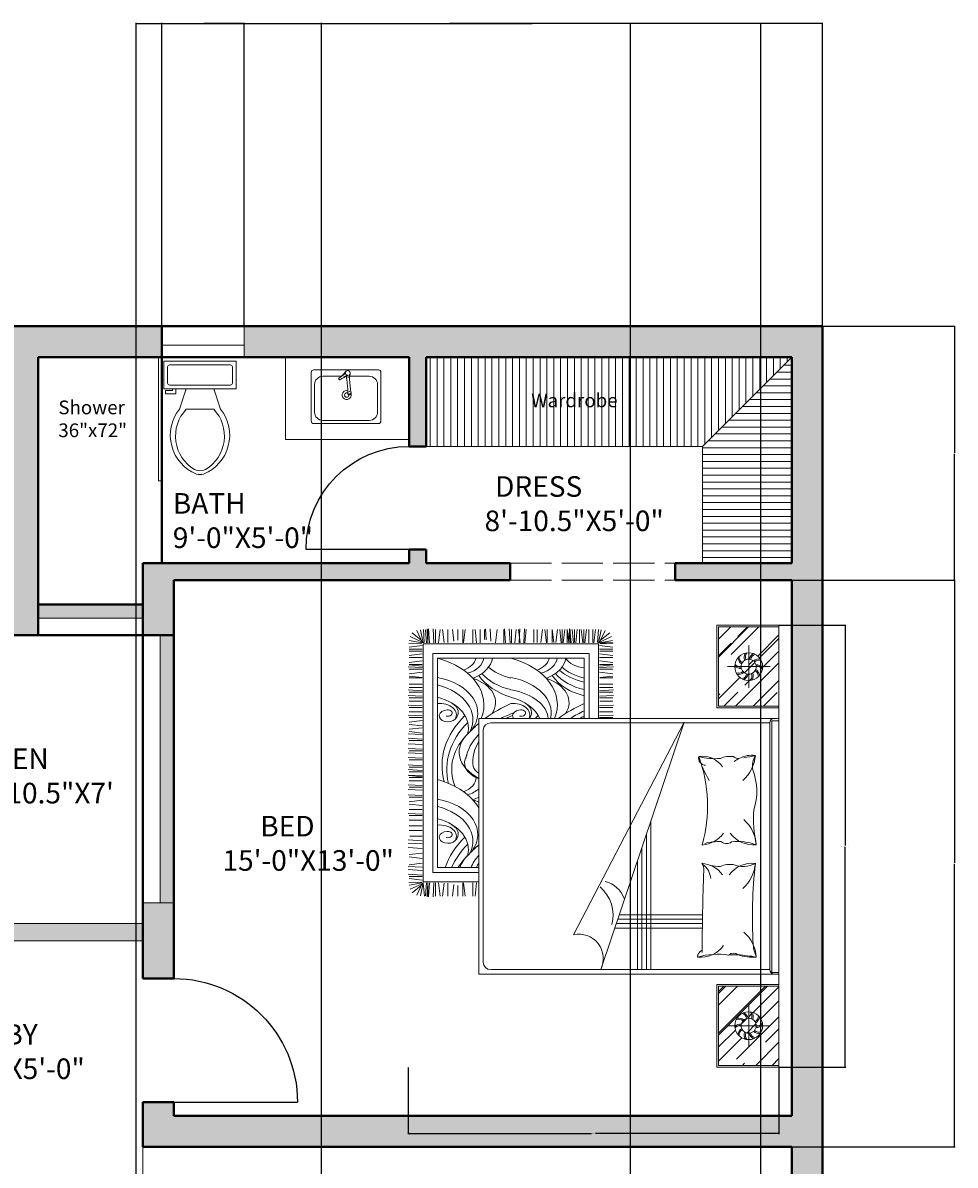
# Model space of a CAD drawing. Units: inches. Extents: x 2985 to 3527, y 3685 to 4528.
# Tile 5 of 5: x 3255 to 3527, y 4195 to 4528. Entities that reach past the tile are written whole.
import ezdxf

# ---------------------------------------------------------------- set-up
doc = ezdxf.new("R2010")
doc.units = ezdxf.units.IN
doc.linetypes.add('ACAD_ISO02W100', pattern=[15, 12, -3])
for name, color, linetype, lineweight in [('A-ANNO-DIMS', 2, 'Continuous', 18), ('A-ANNO-TEXT', 7, 'Continuous', 18), ('A-AREA-IDEN', 7, 'Continuous', 25), ('A-FLOR-CASE', 9, 'Continuous', 20), ('A-FLOR-CASE-PATT', 9, 'Continuous', 13), ('A-FLOR-FIXT', 9, 'Continuous', 18), ('A-FURN', 8, 'Continuous', 18), ('A-GLAZ', 4, 'Continuous', 18), ('A-WALL', 7, 'Continuous', 40), ('A-WALL-OVHD', 7, 'ACAD_ISO02W100', 18), ('A-WALL-PATT', 8, 'Continuous', 13), ('door', 4, 'Continuous', 25)]:
    doc.layers.add(name, color=color, linetype=linetype, lineweight=lineweight)
doc.layers.add('A-GLAZ-PATT', color=241, linetype='Continuous', lineweight=13, true_color=0xf7abae)
doc.styles.get("Standard").update_dxf_attribs({"font": 'arial.ttf'})
doc.dimstyles.get("Standard").update_dxf_attribs({"dimtxt": 0.18, "dimasz": 0.18, "dimexe": 0.18, "dimexo": 0.0625, "dimgap": 0.09, "dimtad": 0, "dimtih": 1, "dimtoh": 1, "dimdec": 4, "dimzin": 0, "dimdsep": 46, "dimtxsty": 'Standard', "dimcen": 0.09, "dimadec": 0, "dimazin": 0, "dimtfac": 1, "dimtdec": 4, "dimtofl": 0, "dimtmove": 0, "dimatfit": 3, "dimfxl": 1, "dimtolj": 1, "dimtzin": 0, "dimarcsym": 0})

# ---------------------------------------------------------------- blocks, each defined once
blk = doc.blocks.new('*U2')
for p, q in [((9.5, -6), (9.5, -2)), ((-10, -8.5), (-8, -8.5)), ((-10, -9.5), (-10, -8.5)), ((-7, -9.5), (-10, -9.5)), ((-8, -8.5), (-8, -8)), ((-7, -8), (-7, -9.5)), ((-4, -8), (-6, -14)), ((4, -8), (6, -14)), ((4, -14), (-4, -14))]:
    blk.add_line(p, q)
blk.add_lwpolyline([(10.5, -8), (10.5, 0), (-10.5, 0), (-10.5, -8)], close=True)
for points in [[(-9.5, -2), (-9.5, -6)], [(8.5, -1), (-8.5, -1)], [(-8.5, -7), (8.5, -7)]]:
    blk.add_lwpolyline(points)
for centre, radius, start, end in [((-8.62, -1.88), 0.884, 81.8699, 188.1301), ((8.62, -1.88), 0.884, 351.8699, 98.1301), ((-8.62, -6.12), 0.884, 171.8699, 278.1301), ((8.62, -6.12), 0.884, 261.8699, 8.1301), ((3.52, -21.58), 12.17, 141.4691, 247.9714), ((4.2, -21.82), 11.33, 136.3677, 238.9468), ((-3.52, -21.58), 12.17, 292.0284, 38.5307), ((-4.2, -21.82), 11.33, 301.053, 43.6321), ((0, -27.88), 4, 245.7318, 294.2682), ((0, -29), 4, 254.8605, 285.1395)]:
    blk.add_arc(centre, radius, start, end)
blk = doc.blocks.new('A$C1B254B08')
for p, q in [((0, 20), (0, 394.5)), ((20, 414.5), (278.5, 414.5)), ((90.2, 364.5), (232.9, 364.5)), ((278.5, 414.5), (518, 414.5)), ((296.4, 364.5), (447.8, 364.5)), ((538, 394.5), (538, 20)), ((26.2, 88.5), (26.2, 300.5)), ((275, 340.3), (282.6, 261.9)), ((303, 263.9), (295.5, 341.4)), ((511.8, 300.5), (511.8, 88.5)), ((447.8, 24.5), (90.2, 24.5)), ((518, 0), (20, 0))]:
    blk.add_line(p, q)
for centre, radius, start, end in [((20, 394.5), 20, 90, 180), ((90.2, 300.5), 64, 90, 180), ((59.9, 551.8), 255, 307.29995, 323.44123), ((362.9, 125.6), 255, 107.37848, 123.51976), ((189.9, 438.1), 86.6, 305.66886, 327.17012), ((298.2, 285.8), 86.6, 103.6496, 125.15085), ((280, 388.4), 16.2, 164.00843, 277.23501), ((280.7, 388), 20, 287.37848, 143.44123), ((175.5, 330.4), 100, 5.6774, 19.04527), ((246.9, 349.5), 29.3, 4.17107, 27.91331), ((320.7, 356.3), 29.3, 157.81042, 186.31744), ((395, 351.3), 100, 162.19035, 185.67746), ((447.8, 300.5), 64, 0, 90), ((518, 394.5), 20, 0, 90), ((218.4, 343.7), 6.64, 127.29995, 303.51976), ((220.3, 343.9), 4.91, 158.92924, 241.9125), ((273.7, 220.2), 34.6, 74.3543, 12.13808), ((273.7, 220.2), 16.8, 61.4601, 4.85789), ((295.6, 234.6), 13.9, 171.17496, 20.1799), ((183.1, 252), 100, 351.17496, 5.6774), ((295.7, 235), 8.12, 213.71984, 15.80061), ((295.2, 239.5), 7.59, 64.48838, 123.74119), ((402.5, 273.8), 100, 185.67746, 200.1799), ((90.2, 88.5), 64, 180, 270), ((447.8, 88.5), 64, 270, 0), ((20, 20), 20, 180, 270), ((518, 20), 20, 270, 0)]:
    blk.add_arc(centre, radius, start, end)
blk = doc.blocks.new('A$C64B41DC1')
for p, q in [((0, 2.5079), (2.9903, 2.5079)), ((0, 2.0879), (0, 2.5079)), ((0.012, 2.4618), (0.0581, 2.5079)), ((0.012, 2.3515), (0.1684, 2.5079)), ((0.012, 2.0999), (0.012, 2.5079)), ((0.0543, 2.2213), (0.3409, 2.5079)), ((0.1689, 2.4179), (0.2589, 2.5079)), ((0.3265, 2.386), (0.4484, 2.5079)), ((0.3699, 2.3332), (0.5445, 2.5079)), ((0.548, 2.5079), (0.548, 2.0999)), ((0.56, 2.5079), (0.56, 2.0879)), ((0.6301, 2.5079), (0.6301, 0.4779)), ((0.6401, 2.461), (0.6401, 2.5079)), ((0.6401, 2.5079), (2.344, 2.5079)), ((2.344, 2.5079), (2.3601, 2.5079)), ((2.344, 2.5079), (2.344, 2.461)), ((2.3601, 2.5079), (2.3601, 2.4761)), ((2.3601, 0.4779), (2.3601, 2.5079)), ((2.4303, 2.5079), (2.4303, 2.0879)), ((2.4423, 2.5079), (2.4423, 2.0999)), ((2.4423, 2.3333), (2.6169, 2.5079)), ((2.4423, 2.2145), (2.7357, 2.5079)), ((2.4423, 2.404), (2.5354, 2.4971)), ((2.705, 2.398), (2.8149, 2.5079)), ((2.7691, 2.3772), (2.8998, 2.5079)), ((2.7819, 2.3646), (2.9252, 2.5079)), ((2.9783, 2.0999), (2.9783, 2.5079)), ((2.9903, 2.0879), (2.9903, 2.5079)), ((0.2157, 2.0999), (0.548, 2.4322)), ((0.2299, 2.0999), (0.548, 2.418)), ((0.2804, 2.1597), (0.2804, 2.4481)), ((2.344, 2.461), (0.6401, 2.461)), ((0.6601, 2.4461), (1.4951, 2.4461)), ((0.6601, 2.4461), (0.6601, 0.5579)), ((1.4951, 2.4461), (0.6697, 2.4461)), ((2.3301, 2.4461), (1.4951, 2.4461)), ((2.3301, 0.5579), (2.3301, 2.4461)), ((2.7099, 2.1597), (2.7099, 2.4481)), ((0.2311, 2.2906), (0.2937, 2.3532)), ((0.3405, 2.3039), (0.3605, 2.3238)), ((2.6158, 2.3088), (2.6313, 2.3243)), ((2.6674, 2.2756), (2.7382, 2.3464)), ((2.7249, 2.3076), (2.7512, 2.3339)), ((2.7914, 2.1846), (2.9783, 2.3715)), ((0.012, 2.261), (0.0275, 2.2765)), ((0.0404, 2.0999), (0.1982, 2.2578)), ((0.1362, 2.3039), (0.4246, 2.3039)), ((0.2905, 2.2539), (0.3304, 2.2938)), ((2.4918, 2.0999), (2.6366, 2.2447)), ((2.8541, 2.3039), (2.5657, 2.3039)), ((2.5849, 2.2779), (2.6158, 2.3088)), ((2.7746, 2.0999), (2.9783, 2.3036)), ((2.9144, 2.2312), (2.9783, 2.2951)), ((0.1365, 2.0999), (0.251, 2.2144)), ((0.4194, 2.0999), (0.548, 2.2285)), ((2.4423, 2.1353), (2.5382, 2.2312)), ((2.7831, 2.0999), (2.8678, 2.1846)), ((2.8962, 2.0999), (2.9783, 2.182)), ((0.56, 2.0879), (0, 2.0879)), ((0.548, 2.0999), (0.012, 2.0999)), ((0.4986, 2.0999), (0.548, 2.1493)), ((0.5127, 2.0999), (0.548, 2.1352)), ((2.4303, 2.0879), (2.9903, 2.0879)), ((2.4423, 2.0999), (2.9783, 2.0999)), ((2.5172, 2.0999), (2.5269, 2.1096)), ((0.9415, 1.9902), (0.9415, 1.3975)), ((0.9715, 1.9906), (0.9715, 1.4076)), ((1.0015, 1.991), (1.0015, 1.4177)), ((1.0315, 1.9916), (1.0315, 1.4279)), ((2.3349, 1.8678), (0.6613, 1.3029)), ((0.8956, 1.1191), (2.3349, 1.8678)), ((1.6636, 1.6412), (0.6601, 1.6412)), ((1.5748, 1.6112), (0.6601, 1.6112)), ((2.3665, 1.295), (2.3665, 1.3839)), ((2.377, 1.295), (2.3822, 1.3891)), ((2.4032, 1.295), (2.4032, 1.3839)), ((2.4346, 1.295), (2.4346, 1.3839)), ((2.4451, 1.295), (2.4503, 1.3891)), ((2.4774, 1.2957), (2.4774, 1.3837)), ((2.5, 1.295), (2.5, 1.3839)), ((2.5105, 1.295), (2.5157, 1.3891)), ((2.5367, 1.295), (2.5367, 1.3839)), ((2.5471, 1.295), (2.5524, 1.3891)), ((2.5681, 1.295), (2.5681, 1.3839)), ((2.5918, 1.295), (2.5918, 1.3839)), ((2.6346, 1.2957), (2.6346, 1.3837)), ((2.6362, 1.2957), (2.6467, 1.3839)), ((2.6729, 1.295), (2.6624, 1.3839)), ((2.6938, 1.295), (2.6938, 1.3839)), ((2.7043, 1.295), (2.7095, 1.3891)), ((2.7127, 1.2957), (2.7232, 1.3839)), ((2.7253, 1.295), (2.7253, 1.3839)), ((2.7494, 1.295), (2.7389, 1.3839)), ((2.7718, 1.295), (2.7718, 1.3839)), ((2.7959, 1.295), (2.7854, 1.3839)), ((2.8146, 1.2957), (2.8146, 1.3837)), ((2.8146, 1.2957), (2.8146, 1.3837)), ((2.8282, 1.295), (2.8282, 1.3839)), ((2.8282, 1.295), (2.8282, 1.3839)), ((2.8523, 1.295), (2.8418, 1.3839)), ((2.8523, 1.295), (2.8418, 1.3839)), ((2.8653, 1.2966), (2.8688, 1.3861)), ((2.8711, 1.2957), (2.8711, 1.3837)), ((2.8711, 1.2957), (2.8875, 1.3822)), ((2.8713, 1.2927), (2.954, 1.3315)), ((2.8765, 1.2958), (2.9132, 1.3758)), ((2.8893, 1.3011), (2.9394, 1.3636)), ((2.3601, 1.2873), (2.8639, 1.2873)), ((2.8639, 1.2873), (2.8639, 0.1018)), ((2.8716, 1.2565), (2.9605, 1.2669)), ((2.8717, 1.2884), (2.9588, 1.3058)), ((2.8723, 1.2489), (2.9603, 1.2489)), ((2.8744, 1.2817), (2.9603, 1.2869)), ((2.3601, 1.2233), (2.7999, 1.2233)), ((2.3601, 1.1913), (2.7679, 1.1912)), ((2.7679, 1.1912), (2.7679, 0.1978)), ((2.7999, 1.2233), (2.7999, 0.1658)), ((2.8716, 1.2212), (2.9605, 1.2212)), ((2.8716, 1.1947), (2.9605, 1.2052)), ((2.8716, 1.181), (2.9605, 1.1705)), ((2.8716, 1.1595), (2.9605, 1.1595)), ((2.8723, 1.1872), (2.9603, 1.1872)), ((2.8716, 1.133), (2.9605, 1.1435)), ((2.8716, 1.1193), (2.9605, 1.1088)), ((2.8716, 1.1035), (2.9605, 1.093)), ((2.8716, 1.0965), (2.9605, 1.0965)), ((2.8716, 1.086), (2.9657, 1.0913)), ((2.8723, 1.1255), (2.9603, 1.1255)), ((2.8723, 1.0858), (2.9605, 1.0753)), ((2.8716, 1.0756), (2.9605, 1.0756)), ((2.8716, 1.0491), (2.9605, 1.0596)), ((2.8716, 1.0354), (2.9605, 1.0249)), ((2.8723, 1.0416), (2.9603, 1.0416)), ((2.8723, 0.9987), (2.9605, 1.0092)), ((2.8716, 0.9346), (2.9605, 0.9241)), ((2.8723, 0.985), (2.9605, 0.9745)), ((2.8723, 0.9735), (2.9603, 0.9735)), ((2.8723, 0.9408), (2.9603, 0.9408)), ((2.8723, 0.8979), (2.9605, 0.9084)), ((2.8723, 0.8726), (2.9603, 0.8726)), ((2.8723, 0.8505), (2.9603, 0.8505)), ((2.8716, 0.7885), (2.9605, 0.799)), ((2.8716, 0.7818), (2.9657, 0.787)), ((2.8716, 0.7503), (2.9657, 0.7556)), ((2.8716, 0.7204), (2.9605, 0.7309)), ((2.8716, 0.6995), (2.9605, 0.6995)), ((2.8723, 0.7571), (2.9605, 0.7466)), ((2.8716, 0.689), (2.9657, 0.6838)), ((2.8716, 0.6576), (2.9657, 0.6523)), ((2.8716, 0.6471), (2.9605, 0.6471)), ((2.8716, 0.5903), (2.9605, 0.6007)), ((2.882, 0.5582), (2.9657, 0.5536)), ((0.6301, 0.4779), (2.3601, 0.4779)), ((0.7101, 0.5079), (2.2801, 0.5079)), ((1.2542, 0.1018), (1.2542, 0.4779)), ((1.3182, 0.1658), (1.3182, 0.4779)), ((1.3502, 0.1978), (1.3502, 0.4779)), ((2.8716, 0.4877), (2.9603, 0.4877)), ((2.8909, 0.5263), (2.9657, 0.5222)), ((2.8928, 0.5169), (2.9605, 0.5169)), ((1.2465, 0.4625), (1.1576, 0.452)), ((1.2465, 0.4365), (1.1577, 0.4365)), ((2.8716, 0.4625), (2.9605, 0.452)), ((2.8716, 0.4365), (2.9603, 0.4365)), ((1.2465, 0.3746), (1.1576, 0.3851)), ((1.2355, 0.3092), (1.1576, 0.3)), ((1.2465, 0.3684), (1.1577, 0.3684)), ((1.2285, 0.3357), (1.1577, 0.3357)), ((2.8716, 0.3746), (2.9605, 0.3851)), ((2.8716, 0.3684), (2.9603, 0.3684)), ((2.8826, 0.3092), (2.9605, 0.3)), ((2.8896, 0.3357), (2.9603, 0.3357)), ((1.2457, 0.2423), (1.1576, 0.2319)), ((1.2457, 0.2676), (1.1577, 0.2676)), ((2.8723, 0.2676), (2.9603, 0.2676)), ((2.8723, 0.2423), (2.9605, 0.2319)), ((1.2465, 0.1742), (1.1524, 0.169)), ((1.2465, 0.2057), (1.1576, 0.2161)), ((1.2465, 0.1847), (1.1576, 0.1847)), ((2.7999, 0.1658), (1.3182, 0.1658)), ((2.7679, 0.1978), (1.3502, 0.1978)), ((2.8716, 0.2057), (2.9605, 0.2161)), ((2.8716, 0.1847), (2.9605, 0.1847)), ((2.8716, 0.1742), (2.9657, 0.169)), ((1.2465, 0.1428), (1.1524, 0.1376)), ((1.2465, 0.1334), (1.1524, 0.1281)), ((1.2465, 0.1323), (1.1576, 0.1323)), ((1.2465, 0.1323), (1.1576, 0.1323)), ((1.2465, 0.1), (1.1576, 0.1105)), ((1.2465, 0.1229), (1.1588, 0.1168)), ((1.2464, 0.1007), (1.1592, 0.0833)), ((1.2468, 0.0964), (1.1641, 0.0576)), ((1.2288, 0.088), (1.1787, 0.0255)), ((1.2415, 0.0933), (1.2049, 0.0133)), ((1.247, 0.0934), (1.2306, 0.0069)), ((1.2527, 0.0925), (1.2493, 0.003)), ((2.8639, 0.1018), (1.2542, 0.1018)), ((1.2658, 0.0941), (1.2762, 0.0052)), ((1.2899, 0.0941), (1.2899, 0.0052)), ((1.2999, 0.0941), (1.3051, 0)), ((1.3313, 0.0941), (1.3365, 0)), ((1.3523, 0.0941), (1.3575, 0)), ((1.3804, 0.0941), (1.3699, 0.0052)), ((1.4119, 0.0934), (1.4223, 0.0052)), ((1.4485, 0.0941), (1.438, 0.0052)), ((1.48, 0.0941), (1.4852, 0)), ((1.5114, 0.0941), (1.5166, 0)), ((1.5323, 0.0941), (1.5376, 0)), ((1.5638, 0.0941), (1.5638, 0.0105)), ((1.6021, 0.0941), (1.6021, 0.0052)), ((1.6336, 0.0941), (1.6336, 0.0052)), ((1.6702, 0.0941), (1.6702, 0.0052)), ((1.7017, 0.0941), (1.7017, 0.0052)), ((1.7122, 0.0941), (1.7174, 0)), ((1.7445, 0.0934), (1.7445, 0.0054)), ((1.7698, 0.0934), (1.7803, 0.0052)), ((1.8065, 0.0941), (1.796, 0.0052)), ((1.8274, 0.0941), (1.8274, 0.0052)), ((1.8379, 0.0941), (1.8431, 0)), ((1.8746, 0.0941), (1.8798, 0)), ((1.8955, 0.0941), (1.8955, 0.0052)), ((1.906, 0.0941), (1.9113, 0)), ((1.9384, 0.0934), (1.9384, 0.0054)), ((1.9609, 0.0941), (1.9609, 0.0052)), ((1.9636, 0.0934), (1.9741, 0.0052)), ((1.9714, 0.0941), (1.9766, 0)), ((1.9976, 0.0941), (1.9976, 0.0052)), ((2.0081, 0.0941), (2.0133, 0)), ((2.029, 0.0941), (2.029, 0.0052)), ((2.0395, 0.0941), (2.0447, 0)), ((2.0797, 0.0941), (2.0797, 0.0052)), ((2.0902, 0.0941), (2.0954, 0)), ((2.1216, 0.0941), (2.1269, 0)), ((2.1412, 0.0941), (2.1412, 0.0052)), ((2.1517, 0.0941), (2.1569, 0)), ((2.1831, 0.0941), (2.1884, 0)), ((2.2093, 0.0941), (2.2093, 0.0052)), ((2.2198, 0.0941), (2.225, 0)), ((2.2512, 0.0941), (2.2565, 0)), ((2.2603, 0.0934), (2.2707, 0.0052)), ((2.2969, 0.0941), (2.2864, 0.0052)), ((2.3089, 0.0934), (2.3193, 0.0052)), ((2.3455, 0.0941), (2.3351, 0.0052)), ((2.3665, 0.0941), (2.3665, 0.0052)), ((2.377, 0.0941), (2.3822, 0)), ((2.4032, 0.0941), (2.4032, 0.0052)), ((2.4346, 0.0941), (2.4346, 0.0052)), ((2.4451, 0.0941), (2.4503, 0)), ((2.4774, 0.0934), (2.4774, 0.0054)), ((2.5, 0.0941), (2.5, 0.0052)), ((2.5105, 0.0941), (2.5157, 0)), ((2.5367, 0.0941), (2.5367, 0.0052)), ((2.5471, 0.0941), (2.5524, 0)), ((2.5681, 0.0941), (2.5681, 0.0052)), ((2.5918, 0.0941), (2.5918, 0.0052)), ((2.6346, 0.0934), (2.6346, 0.0054)), ((2.6362, 0.0934), (2.6467, 0.0052)), ((2.6729, 0.0941), (2.6624, 0.0052)), ((2.6938, 0.0941), (2.6938, 0.0052)), ((2.7043, 0.0941), (2.7095, 0)), ((2.7127, 0.0934), (2.7232, 0.0052)), ((2.7253, 0.0941), (2.7253, 0.0052)), ((2.7494, 0.0941), (2.7389, 0.0052)), ((2.7718, 0.0941), (2.7718, 0.0052)), ((2.7959, 0.0941), (2.7854, 0.0052)), ((2.8146, 0.0934), (2.8146, 0.0054)), ((2.8282, 0.0941), (2.8282, 0.0052)), ((2.8523, 0.0941), (2.8418, 0.0052)), ((2.8653, 0.0925), (2.8688, 0.003)), ((2.8711, 0.0934), (2.8875, 0.0069)), ((2.8713, 0.0964), (2.954, 0.0576)), ((2.8716, 0.1428), (2.9657, 0.1376)), ((2.8716, 0.1334), (2.9657, 0.1281)), ((2.8716, 0.1323), (2.9605, 0.1323)), ((2.8716, 0.1229), (2.9593, 0.1168)), ((2.8717, 0.1007), (2.9588, 0.0833)), ((2.8744, 0.1074), (2.9603, 0.1022)), ((2.8765, 0.0933), (2.9132, 0.0133)), ((2.8893, 0.088), (2.9394, 0.0255))]:
    blk.add_line(p, q)
at = {"ltscale": 10}
for p, q in [((1.4859, 1.5812), (0.6601, 1.5812)), ((1.397, 1.5512), (0.6601, 1.5512))]:
    blk.add_line(p, q, dxfattribs=at)
for centre, radius in [((0.2804, 2.3039), 0.0942), ((2.7099, 2.3039), 0.0942), ((0.2804, 2.3039), 0.051), ((2.7099, 2.3039), 0.051)]:
    blk.add_circle(centre, radius)
for centre, radius, start, end in [((0.6601, 2.4761), 0.03, 180, 270), ((2.3301, 2.4761), 0.03, 270, 0), ((0.3286, 2.3561), 0.0605, 136.17003, 182.48975), ((0.3231, 2.3585), 0.0462, 124.30017, 184.53802), ((2.6672, 2.3585), 0.0462, 355.46198, 55.69983), ((2.6617, 2.3561), 0.0605, 357.51025, 43.82997), ((0.2457, 2.3659), 0.0605, 208.17003, 254.48975), ((0.2417, 2.3614), 0.0462, 196.30017, 256.53802), ((0.2887, 2.3745), 0.0605, 172.17003, 218.48975), ((0.2828, 2.3731), 0.0462, 160.30017, 220.53802), ((0.3501, 2.3178), 0.0605, 100.17003, 146.48975), ((0.347, 2.323), 0.0462, 88.30017, 148.53802), ((0.3449, 2.2742), 0.0605, 64.17003, 110.48975), ((0.3455, 2.2802), 0.0462, 52.30017, 112.53802), ((1.0526, 2.3302), 0.3085, 175.30484, 198.69419), ((-0.8702, 2.0941), 1.6364, 4.80985, 9.18918), ((0.8579, 2.6278), 0.2948, 247.51785, 264.26696), ((0.728, 2.111), 0.245, 40.4189, 85.9871), ((1.0164, 5.7096), 3.3803, 266.81337, 276.16021), ((1.3963, 2.1044), 0.245, 94.0129, 139.5811), ((1.1858, 2.3288), 0.1943, 306.5711, 5.88998), ((1.5348, 2.2652), 0.1767, 151.77364, 201.69827), ((1.6986, 2.3355), 0.1943, 174.11002, 233.4289), ((1.1481, 2.2311), 0.3783, 353.49469, 19.18669), ((1.6871, 3.192), 0.8561, 257.74383, 273.62843), ((1.4882, 2.111), 0.245, 40.4189, 85.9871), ((1.8674, 1.9709), 0.3878, 68.20259, 108.9817), ((2.1269, 2.1044), 0.245, 94.0129, 139.5811), ((2.0342, 2.4856), 0.1563, 261.59582, 298.90918), ((1.9165, 2.3288), 0.1943, 333.73715, 5.88998), ((2.6058, 2.2028), 0.517, 163.60457, 172.3273), ((2.6448, 2.2802), 0.0462, 67.46198, 127.69983), ((2.6454, 2.2742), 0.0605, 69.51025, 115.82997), ((2.6433, 2.323), 0.0462, 31.46198, 91.69983), ((2.6402, 2.3178), 0.0605, 33.51025, 79.82997), ((2.7075, 2.3731), 0.0462, 319.46198, 19.69983), ((2.7016, 2.3745), 0.0605, 321.51025, 7.82997), ((2.7486, 2.3614), 0.0462, 283.46198, 343.69983), ((2.7446, 2.3659), 0.0605, 285.51025, 331.82997), ((0.2153, 2.3276), 0.0462, 232.30017, 292.53802), ((0.2158, 2.3336), 0.0605, 244.17003, 290.48975), ((0.2138, 2.2848), 0.0462, 268.30017, 328.53802), ((0.2107, 2.29), 0.0605, 280.17003, 326.48975), ((0.2377, 2.2493), 0.0462, 304.30017, 4.53802), ((0.2322, 2.2517), 0.0605, 316.17003, 2.48975), ((0.2779, 2.2347), 0.0462, 340.30017, 40.53802), ((0.272, 2.2333), 0.0605, 352.17003, 38.48975), ((0.3191, 2.2464), 0.0462, 16.30017, 76.53802), ((0.3151, 2.2419), 0.0605, 28.17003, 74.48975), ((1.9165, 2.3288), 0.1943, 320.94042, 333.73715), ((2.1347, 2.2313), 0.0459, 165.35061, 223.26844), ((2.6752, 2.2419), 0.0605, 105.51025, 151.82997), ((2.6712, 2.2464), 0.0462, 103.46198, 163.69983), ((2.7182, 2.2333), 0.0605, 141.51025, 187.82997), ((2.7123, 2.2347), 0.0462, 139.46198, 199.69983), ((2.7581, 2.2517), 0.0605, 177.51025, 223.82997), ((2.7526, 2.2493), 0.0462, 175.46198, 235.69983), ((2.7796, 2.29), 0.0605, 213.51025, 259.82997), ((2.7765, 2.2848), 0.0462, 211.46198, 271.69983), ((2.7744, 2.3336), 0.0605, 249.51025, 295.82997), ((2.775, 2.3276), 0.0462, 247.46198, 307.69983), ((0.2688, 2.0945), 0.4956, 344.0243, 8.70709), ((0.7274, 2.2013), 0.0446, 314.4736, 42.17134), ((-1.6008, 2.277), 2.3618, 357.39054, 358.88764), ((1.204, 2.1778), 0.1681, 337.01697, 7.53676), ((1.5671, 2.1546), 0.0547, 142.08329, 220.902), ((1.9346, 2.1778), 0.1681, 337.01697, 7.53676), ((0.9385, 1.978), 0.1943, 126.5711, 185.88998), ((1.1858, 1.9714), 0.1943, 4.31813, 53.4289), ((1.5415, 2.0969), 0.1834, 175.22328, 196.23004), ((1.7059, 1.9714), 0.204, 127.11975, 175.09005), ((1.1965, 2.0983), 0.3299, 343.79543, 3.55541), ((1.9394, 1.991), 0.1651, 351.26213, 55.75721), ((2.4617, 2.0719), 0.3745, 173.82958, 196.4356), ((1.2687, 1.9248), 0.1223, 33.62799, 86.47438), ((1.7676, 1.0629), 0.9631, 69.65065, 105.96307), ((2.2748, 2.5795), 0.6373, 238.34989, 254.31375), ((2.0911, 2.0123), 0.0478, 179.77267, 283.80184), ((0.7417, 2.0149), 0.057, 273.47085, 328.54118), ((0.728, 2.2025), 0.245, 274.0129, 278.34166), ((0.7246, 18.8439), 16.8552, 270.17399, 272.05214), ((1.3401, 1.9404), 0.0603, 49.09906, 101.37023), ((1.0747, 1.2871), 0.1871, 14.1863, 69.12121), ((0.7347, 1.1553), 0.1649, 347.31088, 116.44537), ((1.0274, 1.1334), 0.2527, 40.62904, 104.37123), ((0.7101, 0.5579), 0.05, 180, 270), ((2.2801, 0.5579), 0.05, 270, 0)]:
    blk.add_arc(centre, radius, start, end)
for centre, major_axis, ratio, start_param, end_param in [((1.9938, 1.6262), (0, -0.7531), 0.68, 0.797284, 0.954936), ((2.0643, 1.466), (0, -0.5322), 0.68, 7.239912, 7.311536), ((1.9052, 1.7397), (0, -0.9842), 0.68, 0.74745, 0.979724), ((2.7455, 1.3081), (0, 0.3614), 0.68, 1.900046, 2.742661), ((2.7868, 1.3081), (0, 0.3614), 0.68, 1.900046, 2.614747), ((2.8372, 1.3081), (0, 0.3614), 0.68, 1.900046, 2.479658), ((2.8607, 1.3211), (0, 0.3614), 0.68, 1.938265, 2.479658), ((2.8057, 1.2079), (0, -0.1524), 0.68, 4.821745, 5.895886), ((2.4665, 0.8216), (0, -0.2664), 0.68, 2.006169, 3.565187), ((2.4513, 0.5069), (0, 0.502), 0.68, 5.095327, 6.553458), ((2.7862, 0.8069), (0, -0.2615), 0.68, 3.244645, 4.205018), ((2.7784, 0.8289), (0, -0.1802), 0.68, 3.227058, 4.318474), ((2.396, 0.6032), (0, 0.3641), 0.68, -1.3172, 0.145284), ((2.3507, 0.5642), (0.0073, 0.3819), 0.56205, -1.21172, -0.009991), ((2.7821, 0.7971), (0, -0.1589), 0.68, 3.272942, 4.229533), ((2.2964, 0.5771), (0, -0.3263), 0.68, 1.938944, 2.850232), ((2.0403, 1.6015), (0, -0.8763), 0.68, 6.849801, 6.887077), ((2.4005, 0.7132), (0, -0.1214), 0.68, 2.284368, 3.652258), ((2.3834, 0.7081), (0, 0.1147), 0.68, 4.593909, 6.585576), ((2.3961, 0.7628), (0, -0.0317), 0.68, 1.462497, 5.046281), ((2.3774, 0.7653), (0, -0.0593), 0.68, 5.841311, 7.755362), ((1.9938, 1.1295), (-0.0678, 0.7439), 0.610498, 3.917146, 4.063997), ((2.0643, 0.9693), (0, -0.5322), 0.68, 7.239912, 7.336618), ((1.9052, 1.243), (0, -0.9842), 0.68, 0.74745, 0.979724), ((2.4665, 0.3249), (0, -0.2664), 0.68, 2.006169, 3.565187), ((2.7455, 0.8114), (-0.0599, 0.3735), 0.695517, 1.775813, 2.548612), ((2.7868, 0.8114), (0, 0.3614), 0.68, 1.900046, 2.614747), ((2.8607, 0.8243), (0, 0.3614), 0.68, 1.938265, 2.479658), ((2.4513, 0.0102), (0, 0.502), 0.68, 5.095327, 6.553458), ((2.7862, 0.3102), (0, -0.2615), 0.68, 3.244645, 4.205018), ((1.242, 0.9693), (0, -0.5322), 0.68, 6.586764, 6.677612), ((1.1714, 1.1295), (-0.1157, 0.7241), 0.59432, 3.291697, 3.50733), ((1.0828, 1.243), (0, -0.9842), 0.68, 0.565948, 0.680366), ((1.5283, 0.0674), (0, -0.3703), 0.68, 1.930561, 3.464283), ((1.5736, 0.1065), (0, 0.3641), 0.68, -1.3172, 0.476403), ((1.6289, 0.0102), (0, 0.502), 0.68, 6.655152, 6.661293), ((1.6289, 0.0102), (0, 0.502), 0.68, 5.095327, 5.911219), ((1.6442, 0.3249), (0, -0.2664), 0.68, 2.006169, 2.182797), ((1.9638, 0.3102), (0, -0.2615), 0.68, 4.015924, 4.205018), ((1.956, 0.3322), (0, -0.1802), 0.68, 3.770744, 4.318474), ((2.0606, 0.5616), (0, -0.1803), 0.68, 5.194792, 5.929328), ((2.0606, 0.5616), (0, -0.1803), 0.68, 5.194792, 6.723255), ((2.1315, 0.6603), (0, -0.3155), 0.68, 5.328638, 6.949396), ((2.0549, 0.5656), (0, -0.1303), 0.68, 5.450951, 6.054641), ((2.0643, 0.9693), (0, -0.5322), 0.68, 6.20013, 6.677612), ((1.9938, 1.1295), (-0.0678, 0.7439), 0.610498, 3.199135, 3.592282), ((1.9052, 1.243), (0, -0.9842), 0.68, 0.565948, 0.680366), ((2.3507, 0.0674), (0, -0.3703), 0.68, 1.930561, 3.464283), ((2.396, 0.1065), (0, 0.3641), 0.68, -1.3172, 0.476403), ((2.4513, 0.0102), (0, 0.502), 0.68, 6.655152, 6.661293), ((2.7784, 0.3322), (0, -0.1802), 0.68, 3.227058, 4.318474), ((1.1933, 0.9181), (0, -0.624), 0.68, 0.378672, 0.625379), ((1.3091, 0.6603), (0, -0.3155), 0.68, 6.475719, 6.949396), ((1.1911, 1.1066), (0, 0.8458), 0.68, 3.421828, 3.728616), ((1.474, 0.0804), (0, -0.3263), 0.68, 1.938944, 3.339184), ((1.9597, 0.3004), (0, -0.1589), 0.68, 3.14258, 4.229533), ((2.0157, 0.9181), (0, -0.624), 0.68, -0.280078, 0.625379), ((2.0135, 1.1066), (0, 0.8458), 0.68, 2.978727, 3.728616), ((2.2964, 0.0804), (0, -0.3263), 0.68, 1.938944, 3.339184), ((2.7821, 0.3004), (0, -0.1589), 0.68, 3.272942, 4.229533), ((1.2179, 1.1047), (0, -0.8763), 0.68, 6.507006, 6.887077), ((1.555, 0.2685), (0, -0.0593), 0.68, 3.732151, 7.755362), ((1.5781, 0.2165), (0, -0.1214), 0.68, 2.284368, 3.726131), ((1.561, 0.2114), (0, 0.1147), 0.68, 4.593909, 6.647252), ((2.0403, 1.1047), (0, -0.8763), 0.68, 6.099302, 6.887077), ((2.3774, 0.2685), (0, -0.0593), 0.68, 3.732151, 7.755362), ((2.4005, 0.2165), (0, -0.1214), 0.68, 2.284368, 3.726131), ((2.3834, 0.2114), (0, 0.1147), 0.68, 4.593909, 6.647252), ((1.5737, 0.2661), (0, -0.0317), 0.68, 1.462497, 5.046281), ((2.3961, 0.2661), (0, -0.0317), 0.68, 1.462497, 5.046281)]:
    blk.add_ellipse(centre, major_axis=major_axis, ratio=ratio, start_param=start_param, end_param=end_param)
blk = doc.blocks.new('DOOR-SWING-30IN')
blk.add_line((0, 0), (30, 0))
blk.add_arc((0, 0), 30, 0, 90)
blk = doc.blocks.new('DOOR-SWING-36IN')
blk.add_line((0, 0), (0, 36))
blk.add_arc((0, 0), 36, 0, 90)
blk = doc.blocks.new('SHOWER-SCREEN-36IN')
for p in [(1, 36), (0, 0)]:
    blk.add_line(p, (1, 0))
blk = doc.blocks.new('VANITY-TOP-36X24IN')
for p in [(36, 24), (0, 0)]:
    blk.add_line(p, (36, 0))
blk = doc.blocks.new('*D24')
at = {"layer": 'A-ANNO-DIMS', "color": 0, "lineweight": -2, "transparency": 16777216}
for p, q in [((3475.64, 4352.29), (3495.07, 4352.29)), ((3494.89, 4352.11), (3494.89, 4288.1)), ((3494.89, 4223.73), (3494.89, 4287.74)), ((3475.64, 4223.55), (3495.07, 4223.55))]:
    blk.add_line(p, q, dxfattribs=at)
at = {"layer": 'A-ANNO-DIMS', "color": 0, "transparency": 16777216}
for points in [[(3494.86, 4352.11), (3494.92, 4352.11), (3494.89, 4352.29)], [(3494.86, 4223.73), (3494.92, 4223.73), (3494.89, 4223.55)]]:
    blk.add_solid(points, dxfattribs=at)
at = {"layer": 'Defpoints', "color": 0, "transparency": 16777216}
for p in [(3475.58, 4352.29), (3494.89, 4352.29), (3475.58, 4223.55)]:
    blk.add_point(p, dxfattribs=at)
at = {"layer": 'A-ANNO-DIMS', "color": 0, "transparency": 16777216, "insert": (3494.89, 4287.92), "char_height": 0.18, "attachment_point": 5}
blk.add_mtext('\\A1;BED GROUP 129 TYP.', dxfattribs=at)
blk = doc.blocks.new('*D25')
at = {"layer": 'A-ANNO-DIMS', "color": 0, "lineweight": -2, "transparency": 16777216}
for p, q in [((3367.61, 4223.49), (3367.61, 4204.06)), ((3475.58, 4223.49), (3475.58, 4204.06)), ((3367.79, 4204.24), (3421, 4204.24)), ((3475.4, 4204.24), (3422.18, 4204.24))]:
    blk.add_line(p, q, dxfattribs=at)
at = {"layer": 'A-ANNO-DIMS', "color": 0, "transparency": 16777216}
for points in [[(3367.79, 4204.27), (3367.79, 4204.21), (3367.61, 4204.24)], [(3475.4, 4204.27), (3475.4, 4204.21), (3475.58, 4204.24)]]:
    blk.add_solid(points, dxfattribs=at)
at = {"layer": 'Defpoints', "color": 0, "transparency": 16777216}
for p in [(3367.61, 4223.55), (3475.58, 4223.55), (3475.58, 4204.24)]:
    blk.add_point(p, dxfattribs=at)
at = {"layer": 'A-ANNO-DIMS', "color": 0, "transparency": 16777216, "insert": (3421.59, 4204.24), "char_height": 0.18, "attachment_point": 5}
blk.add_mtext('\\A1;108 TYP.', dxfattribs=at)
blk = doc.blocks.new('*D42')
at = {"layer": 'A-ANNO-DIMS', "color": 0, "lineweight": -2, "transparency": 16777216}
for p, q in [((3288.33, 3741.43), (3288.33, 4527.76)), ((3288.51, 4527.58), (3379.05, 4527.58)), ((3470.15, 4527.58), (3379.61, 4527.58)), ((3470.33, 3741.43), (3470.33, 4527.76))]:
    blk.add_line(p, q, dxfattribs=at)
at = {"layer": 'A-ANNO-DIMS', "color": 0, "transparency": 16777216}
for points in [[(3288.51, 4527.61), (3288.51, 4527.55), (3288.33, 4527.58)], [(3470.15, 4527.61), (3470.15, 4527.55), (3470.33, 4527.58)]]:
    blk.add_solid(points, dxfattribs=at)
at = {"layer": 'Defpoints', "color": 0, "transparency": 16777216}
for p in [(3470.33, 4527.58), (3288.33, 3741.37), (3470.33, 3741.37)]:
    blk.add_point(p, dxfattribs=at)
at = {"layer": 'A-ANNO-DIMS', "color": 0, "transparency": 16777216, "insert": (3379.33, 4527.58), "char_height": 0.18, "attachment_point": 5}
blk.add_mtext('\\A1;182', dxfattribs=at)
blk = doc.blocks.new('*D44')
at = {"layer": 'A-ANNO-DIMS', "color": 0, "lineweight": -2, "transparency": 16777216}
for p, q in [((3479.4, 4365.37), (3526.91, 4365.37)), ((3526.73, 4365.19), (3526.73, 4283.05)), ((3526.73, 4200.55), (3526.73, 4282.69)), ((3479.4, 4200.37), (3526.91, 4200.37))]:
    blk.add_line(p, q, dxfattribs=at)
at = {"layer": 'A-ANNO-DIMS', "color": 0, "transparency": 16777216}
for points in [[(3526.7, 4365.19), (3526.76, 4365.19), (3526.73, 4365.37)], [(3526.7, 4200.55), (3526.76, 4200.55), (3526.73, 4200.37)]]:
    blk.add_solid(points, dxfattribs=at)
at = {"layer": 'Defpoints', "color": 0, "transparency": 16777216}
for p in [(3479.33, 4365.37), (3526.73, 4365.37), (3479.33, 4200.37)]:
    blk.add_point(p, dxfattribs=at)
at = {"layer": 'A-ANNO-DIMS', "color": 0, "transparency": 16777216, "insert": (3526.73, 4282.87), "char_height": 0.18, "attachment_point": 5}
blk.add_mtext('\\A1;165', dxfattribs=at)
blk = doc.blocks.new('*D45')
at = {"layer": 'A-ANNO-DIMS', "color": 0, "lineweight": -2, "transparency": 16777216}
for p, q in [((3488.395987, 4439.371951), (3526.913487, 4439.371951)), ((3526.733487, 4439.191951), (3526.733487, 4402.551951)), ((3526.733487, 4365.551951), (3526.733487, 4402.191951)), ((3479.395987, 4365.371951), (3526.913487, 4365.371951))]:
    blk.add_line(p, q, dxfattribs=at)
at = {"layer": 'A-ANNO-DIMS', "color": 0, "transparency": 16777216}
for points in [[(3526.703487, 4439.191951), (3526.763487, 4439.191951), (3526.733487, 4439.371951)], [(3526.703487, 4365.551951), (3526.763487, 4365.551951), (3526.733487, 4365.371951)]]:
    blk.add_solid(points, dxfattribs=at)
at = {"layer": 'Defpoints', "color": 0, "transparency": 16777216}
for p in [(3488.333487, 4439.371951), (3526.733487, 4439.371951), (3479.333487, 4365.371951)]:
    blk.add_point(p, dxfattribs=at)
at = {"layer": 'A-ANNO-DIMS', "color": 0, "transparency": 16777216, "insert": (3526.733487, 4402.371951), "char_height": 0.18, "attachment_point": 5}
blk.add_mtext('\\A1;74', dxfattribs=at)
blk = doc.blocks.new('*D48')
at = {"layer": 'A-ANNO-DIMS', "color": 0, "lineweight": -2, "transparency": 16777216}
for p, q in [((3295.83, 4439.43), (3295.83, 4527.76)), ((3296.01, 4527.58), (3307.61, 4527.58)), ((3319.65, 4527.58), (3308.05, 4527.58)), ((3319.83, 4439.43), (3319.83, 4527.76))]:
    blk.add_line(p, q, dxfattribs=at)
at = {"layer": 'A-ANNO-DIMS', "color": 0, "transparency": 16777216}
for points in [[(3296.01, 4527.61), (3296.01, 4527.55), (3295.83, 4527.58)], [(3319.65, 4527.61), (3319.65, 4527.55), (3319.83, 4527.58)]]:
    blk.add_solid(points, dxfattribs=at)
at = {"layer": 'Defpoints', "color": 0, "transparency": 16777216}
for p in [(3319.83, 4527.58), (3295.83, 4439.37), (3319.83, 4439.37)]:
    blk.add_point(p, dxfattribs=at)
at = {"layer": 'A-ANNO-DIMS', "color": 0, "transparency": 16777216, "insert": (3307.83, 4527.58), "char_height": 0.18, "attachment_point": 5}
blk.add_mtext('\\A1;24', dxfattribs=at)
blk = doc.blocks.new('*D49')
at = {"layer": 'A-ANNO-DIMS', "color": 0, "lineweight": -2, "transparency": 16777216}
for p, q in [((3319.83, 4439.43), (3319.83, 4527.76)), ((3320.01, 4527.58), (3403.7, 4527.58)), ((3488.15, 4527.58), (3404.47, 4527.58)), ((3488.33, 4439.43), (3488.33, 4527.76))]:
    blk.add_line(p, q, dxfattribs=at)
at = {"layer": 'A-ANNO-DIMS', "color": 0, "transparency": 16777216}
for points in [[(3320.01, 4527.61), (3320.01, 4527.55), (3319.83, 4527.58)], [(3488.15, 4527.61), (3488.15, 4527.55), (3488.33, 4527.58)]]:
    blk.add_solid(points, dxfattribs=at)
at = {"layer": 'Defpoints', "color": 0, "transparency": 16777216}
for p in [(3488.33, 4527.58), (3319.83, 4439.37), (3488.33, 4439.37)]:
    blk.add_point(p, dxfattribs=at)
at = {"layer": 'A-ANNO-DIMS', "color": 0, "transparency": 16777216, "insert": (3404.08, 4527.58), "char_height": 0.18, "attachment_point": 5}
blk.add_mtext('\\A1;168.5', dxfattribs=at)
blk = doc.blocks.new('*D53')
at = {"layer": 'A-ANNO-DIMS', "color": 0, "lineweight": -2, "transparency": 16777216}
for p, q in [((3342.33, 4015.43), (3342.33, 4527.76)), ((3342.51, 4527.58), (3387.11, 4527.58)), ((3432.15, 4527.58), (3387.55, 4527.58)), ((3432.33, 4015.43), (3432.33, 4527.76))]:
    blk.add_line(p, q, dxfattribs=at)
at = {"layer": 'A-ANNO-DIMS', "color": 0, "transparency": 16777216}
for points in [[(3342.51, 4527.61), (3342.51, 4527.55), (3342.33, 4527.58)], [(3432.15, 4527.61), (3432.15, 4527.55), (3432.33, 4527.58)]]:
    blk.add_solid(points, dxfattribs=at)
at = {"layer": 'Defpoints', "color": 0, "transparency": 16777216}
for p in [(3432.33, 4527.58), (3342.33, 4015.37), (3432.33, 4015.37)]:
    blk.add_point(p, dxfattribs=at)
at = {"layer": 'A-ANNO-DIMS', "color": 0, "transparency": 16777216, "insert": (3387.33, 4527.58), "char_height": 0.18, "attachment_point": 5}
blk.add_mtext('\\A1;90', dxfattribs=at)

msp = doc.modelspace()

# ---------------------------------------------------------------- hatches: boundary and pattern name
at = {"layer": 'A-FLOR-CASE-PATT'}
h = msp.add_hatch(dxfattribs=at)
h.set_pattern_fill('ANSI31', color=256, scale=0.6299213, angle=45, style=0)
h.paths.add_polyline_path([(3372.833, 4404.372), (3453.333, 4404.372), (3479.333, 4430.372), (3372.833, 4430.372)])
h = msp.add_hatch(dxfattribs=at)
h.set_pattern_fill('ANSI31', color=256, scale=0.6299213, angle=-45, style=0)
h.paths.add_polyline_path([(3453.333, 4370.372), (3479.333, 4370.372), (3479.333, 4430.372), (3453.333, 4404.372)])
at = {"layer": 'A-GLAZ-PATT'}
h = msp.add_hatch(color=256, dxfattribs=at)
h.dxf.hatch_style = 1
h.paths.add_polyline_path([(3216.833, 4349.372), (3212.833, 4349.372), (3212.833, 4271.372), (3216.833, 4271.372)])
h.paths.add_polyline_path([(3250.833, 4358.372), (3221.833, 4358.372), (3221.833, 4354.372), (3250.833, 4354.372)])
h.paths.add_polyline_path([(3290.333, 4358.372), (3259.833, 4358.372), (3259.833, 4354.372), (3290.333, 4354.372)])
h.paths.add_polyline_path([(3299.333, 4349.372), (3295.333, 4349.372), (3295.333, 4271.372), (3299.333, 4271.372)])
h.paths.add_polyline_path([(3290.333, 4265.372), (3221.833, 4265.372), (3221.833, 4260.372), (3290.333, 4260.372)])
at = {"layer": 'A-WALL-PATT'}
h = msp.add_hatch(color=256, dxfattribs=at)
h.dxf.hatch_style = 1
h.paths.add_polyline_path([(3259.833, 4430.372), (3295.833, 4430.372), (3295.833, 4439.372), (3214.833, 4439.372), (3214.833, 4430.372), (3250.833, 4430.372), (3250.833, 4349.372), (3259.833, 4349.372)])
h = msp.add_hatch(color=256, dxfattribs=at)
h.dxf.hatch_style = 1
h.paths.add_polyline_path([(3488.333, 4439.372), (3319.833, 4439.372), (3319.833, 4430.372), (3367.833, 4430.372), (3367.833, 4404.372), (3372.833, 4404.372), (3372.833, 4430.372), (3479.333, 4430.372), (3479.333, 4370.372), (3453.333, 4370.372), (3445.333, 4370.372), (3445.333, 4365.372), (3479.333, 4365.372), (3479.333, 4209.372), (3299.333, 4209.372), (3299.333, 4213.372), (3290.333, 4213.372), (3290.333, 4200.372), (3479.333, 4200.372), (3479.333, 4020.372), (3342.333, 4020.372), (3342.333, 4015.372), (3432.333, 4015.372), (3432.333, 3965.372), (3437.333, 3965.372), (3437.333, 4015.372), (3479.333, 4015.372), (3479.333, 3931.372), (3473.333, 3931.372), (3473.333, 3922.372), (3488.333, 3922.372)])
h = msp.add_hatch(color=256, dxfattribs=at)
h.dxf.hatch_style = 1
h.paths.add_polyline_path([(3397.333, 4370.372), (3372.833, 4370.372), (3372.833, 4374.372), (3367.833, 4374.372), (3367.833, 4370.372), (3290.333, 4370.372), (3290.333, 4349.372), (3299.333, 4349.372), (3299.333, 4365.372), (3397.333, 4365.372)])
h = msp.add_hatch(color=256, dxfattribs=at)
h.dxf.hatch_style = 1
h.paths.add_polyline_path([(3221.833, 4271.372), (3212.833, 4271.372), (3212.833, 4237.372), (3221.833, 4237.372)])
h.paths.add_polyline_path([(3299.333, 4271.372), (3290.333, 4271.372), (3290.333, 4249.372), (3299.333, 4249.372)])

# ---------------------------------------------------------------- linework, layer by layer
at = {"layer": 'A-FLOR-CASE'}
for p, q in [((3453.333, 4404.372), (3479.333, 4430.372)), ((3453.333, 4430.372), (3479.333, 4430.372)), ((3372.833, 4404.372), (3453.333, 4404.372)), ((3453.333, 4404.372), (3453.333, 4370.372))]:
    msp.add_line(p, q, dxfattribs=at)
at = {"layer": 'A-GLAZ'}
for p, q in [((3319.833, 4439.372), (3319.833, 4430.372)), ((3319.833, 4433.872), (3295.833, 4433.872)), ((3259.833, 4354.372), (3290.333, 4354.372)), ((3295.333, 4349.372), (3295.333, 4271.372)), ((3290.333, 4271.372), (3299.333, 4271.372)), ((3221.833, 4265.372), (3290.333, 4265.372)), ((3221.833, 4260.372), (3290.333, 4260.372))]:
    msp.add_line(p, q, dxfattribs=at)
at = {"layer": 'A-WALL'}
for p, q in [((3023.833, 4439.372), (3488.333, 4439.372)), ((3295.833, 4439.372), (3295.833, 4370.372)), ((3488.333, 4439.372), (3488.333, 3922.372)), ((3259.833, 4430.372), (3259.833, 4349.372)), ((3259.833, 4430.372), (3367.833, 4430.372)), ((3367.833, 4430.372), (3367.833, 4404.372)), ((3372.833, 4430.372), (3479.333, 4430.372)), ((3372.833, 4430.372), (3372.833, 4404.372)), ((3479.333, 4430.372), (3479.333, 4370.372)), ((3367.833, 4404.372), (3372.833, 4404.372)), ((3367.833, 4374.372), (3372.833, 4374.372)), ((3367.833, 4374.372), (3367.833, 4370.372)), ((3372.833, 4374.372), (3372.833, 4370.372)), ((3290.333, 4370.372), (3290.333, 4349.372)), ((3290.333, 4370.372), (3367.833, 4370.372)), ((3372.833, 4370.372), (3397.333, 4370.372)), ((3397.333, 4370.372), (3397.333, 4365.372)), ((3445.333, 4370.372), (3445.333, 4365.372)), ((3445.333, 4370.372), (3479.333, 4370.372)), ((3453.333, 4370.372), (3479.333, 4370.372)), ((3299.333, 4365.372), (3397.333, 4365.372)), ((3299.333, 4365.372), (3299.333, 4249.372)), ((3445.333, 4365.372), (3479.333, 4365.372)), ((3479.333, 4365.372), (3479.333, 4209.372)), ((3259.833, 4358.372), (3290.333, 4358.372)), ((3212.833, 4349.372), (3299.333, 4349.372)), ((3290.333, 4349.372), (3290.333, 4249.372)), ((3290.333, 4249.372), (3299.333, 4249.372)), ((3290.333, 4213.372), (3299.333, 4213.372)), ((3290.333, 4213.372), (3290.333, 4200.372)), ((3299.333, 4213.372), (3299.333, 4209.372)), ((3299.333, 4209.372), (3479.333, 4209.372)), ((3290.333, 4200.372), (3479.333, 4200.372)), ((3479.333, 4200.372), (3479.333, 4020.372))]:
    msp.add_line(p, q, dxfattribs=at)
at = {"layer": 'A-WALL-OVHD'}
for p, q in [((3397.333, 4370.372), (3445.333, 4370.372)), ((3397.333, 4365.372), (3445.333, 4365.372)), ((3290.333, 4200.372), (3290.333, 4026.372))]:
    msp.add_line(p, q, dxfattribs=at)

# ---------------------------------------------------------------- block references
at = {"layer": 'A-FLOR-CASE', "extrusion": (0, 0, -1), "zscale": -1}
msp.add_blockref('VANITY-TOP-36X24IN', (-3367.834, 4406.372), dxfattribs=at)
at = {"layer": 'A-FLOR-FIXT', "extrusion": (0, 0, -1), "zscale": -1}
msp.add_blockref('SHOWER-SCREEN-36IN', (-3295.834, 4394.372), dxfattribs=at)
at = {"layer": 'A-FLOR-FIXT'}
msp.add_blockref('*U2', (3306.94, 4429.183), dxfattribs=at)
at = {"layer": 'A-FLOR-FIXT', "xscale": 0.0377799968595654, "yscale": 0.0377799968595654, "zscale": 0.0377799968595654}
msp.add_blockref('A$C1B254B08', (3339.331, 4411.029), dxfattribs=at)
at = {"layer": 'A-FURN', "xscale": -43.05186407285219, "yscale": 43.05186407285219, "zscale": 43.05186407285219, "rotation": 270.0000000000047}
msp.add_blockref('A$C64B41DC1', (3367.607, 4223.551), dxfattribs=at)
at = {"layer": 'door', "extrusion": (0, 0, -1), "zscale": -1}
msp.add_blockref('DOOR-SWING-30IN', (-3367.833, 4374.372), dxfattribs=at)
at = {"layer": 'door', "extrusion": (0, 0, -1), "zscale": -1, "rotation": 90.00000000000254}
msp.add_blockref('DOOR-SWING-36IN', (-3299.333, 4213.372), dxfattribs=at)

# ---------------------------------------------------------------- texts
at = {"layer": 'A-ANNO-TEXT', "char_height": 4, "attachment_point": 1}
for s, width, insert in [('Wardrobe', 30.56793, (3403.417, 4419.784)), ('Shower\\P36"x72"', 31.52609, (3265.671, 4417.739))]:
    msp.add_mtext_dynamic_manual_height_columns(s, width=width, gutter_width=12.5, heights=[0], dxfattribs=dict(at, insert=insert))
at = {"layer": 'A-AREA-IDEN', "attachment_point": 1}
for s, width, insert, char_height in [('    {\\H2.4x;DRESS\\P8\'-10.5"X5\'-0"}', 78.32659, (3389.839, 4395.699), 2.5), ('BATH\\P9\'-0"X5\'-0"', 24.98129, (3299.023, 4390.779), 6), ('OPEN \\P4\'-10.5"X7\'', 31.7894, (3240.887, 4316.386), 6), ('      BED\\P15\'-0"X13\'-0"', 31.99995, (3313.49, 4296.759), 6), ('  {\\H2.4x;LOBBY\\P5\'-3"X5\'-0"}', 56.03015, (3232.521, 4236.086), 2.5)]:
    msp.add_mtext_dynamic_manual_height_columns(s, width=width, gutter_width=12.5, heights=[0], dxfattribs=dict(at, insert=insert, char_height=char_height))

# ---------------------------------------------------------------- dimensions: what is measured, and where the dimension line sits
at = {"layer": 'A-ANNO-DIMS'}
for base, p1, p2, override, picture, middle in [((3470.333, 4527.583), (3288.333, 3741.372), (3470.333, 3741.372), {"dimdec": 0, "dimlfac": 1, "dimrnd": 0, "dimzin": 0, "dimdsep": 46, "dimlunit": 2}, '*D42', (3379.333, 4527.583)), ((3319.833, 4527.583), (3295.833, 4439.372), (3319.833, 4439.372), {"dimdec": 0, "dimlfac": 1, "dimrnd": 0, "dimzin": 0, "dimdsep": 46, "dimlunit": 2}, '*D48', (3307.833, 4527.583)), ((3488.333, 4527.583), (3319.833, 4439.372), (3488.333, 4439.372), {"dimdec": 1, "dimlfac": 1, "dimrnd": 0, "dimzin": 0, "dimdsep": 46, "dimlunit": 2}, '*D49', (3404.083, 4527.583)), ((3432.333, 4527.583), (3342.333, 4015.372), (3432.333, 4015.372), {"dimdec": 0, "dimlfac": 1, "dimrnd": 0, "dimzin": 0, "dimdsep": 46, "dimlunit": 2}, '*D53', (3387.333, 4527.583))]:
    dim = msp.add_linear_dim(base=base, p1=p1, p2=p2, dimstyle='Standard', override=override, dxfattribs=at)
    dim.commit()
    dim.dimension.update_dxf_attribs({"geometry": picture, "text_midpoint": middle})
for base, p1, p2, picture, middle in [((3526.733, 4439.372), (3479.333, 4365.372), (3488.333, 4439.372), '*D45', (3526.733, 4402.372)), ((3526.733, 4365.372), (3479.333, 4200.372), (3479.333, 4365.372), '*D44', (3526.733, 4282.872))]:
    dim = msp.add_linear_dim(base=base, p1=p1, p2=p2, angle=90, dimstyle='Standard', override={"dimdec": 0, "dimlfac": 1, "dimrnd": 0, "dimzin": 0, "dimdsep": 46, "dimlunit": 2}, dxfattribs=at)
    dim.commit()
    dim.dimension.update_dxf_attribs({"geometry": picture, "text_midpoint": middle})
for base, p1, p2, angle, text, picture, middle in [((3494.888, 4352.288), (3475.577, 4223.551), (3475.577, 4352.288), 90, 'BED GROUP <> TYP.', '*D24', (3494.888, 4287.919)), ((3475.577, 4204.24), (3367.607, 4223.551), (3475.577, 4223.551), 0, '<> TYP.', '*D25', (3421.592, 4204.24))]:
    dim = msp.add_linear_dim(base=base, p1=p1, p2=p2, angle=angle, text=text, dimstyle='Standard', override={"dimdec": 0, "dimlfac": 1, "dimrnd": 0, "dimzin": 0, "dimdsep": 46, "dimlunit": 2}, dxfattribs=at)
    dim.commit()
    dim.dimension.update_dxf_attribs({"geometry": picture, "text_midpoint": middle})

doc.saveas('drawing.dxf')
